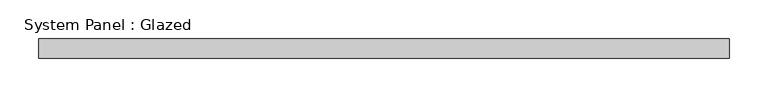
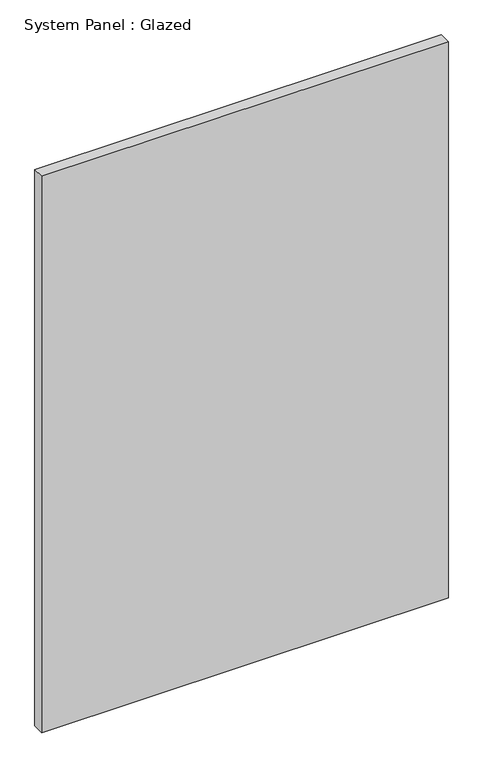
"""IFC4 building model written with IfcOpenShell, lengths in millimetres: plate geometry, System Panel : Glazed."""

from ifc_helpers import new_model, si_unit, origin, origin_with_axes, place, context, project, spatial, polyline, outline, extrude, source, transform, mapped, element, save


def system_panel_glazed_e669d95e(model_context):
    return source(origin(), model_context, "Body", "SweptSolid", [
        extrude(outline(polyline([(447.675, 19.05), (-447.675, 19.05), (-447.675, 44.45), (447.675, 44.45), (447.675, 19.05)])), origin_with_axes(), (0.0, 0.0, 1.0), 1295.1292854),
    ])


if __name__ == "__main__":
    model = new_model("IFC4")
    model_context = context("Model", 3, world=origin())
    ifc_project = project(units=[si_unit("LENGTHUNIT", "METRE", prefix="MILLI")], contexts=[model_context])
    site = spatial("IfcSite", under=ifc_project)
    building = spatial("IfcBuilding", under=site)
    placement = place(None, origin())
    system_panel_glazed_shape = system_panel_glazed_e669d95e(model_context)
    element("IfcPlate", 1, ObjectType="System Panel : Glazed", at=placement, inside=building, context=model_context, shape_type="MappedRepresentation", body=[
        mapped(system_panel_glazed_shape, transform((0.0, 0.0, 0.0), x_axis=(1.0, 0.0, 0.0), y_axis=(0.0, 1.0, 0.0), z_axis=(0.0, 0.0, 1.0))),
    ])
    save(model, "model.ifc")

# Revit data of these elements
# Type "System Panel : Glazed"
#   Construction Type Id = "GSP4R"
#   Analytic Construction = "1/8 in Pilkington single glazing"
#   Visual Light Transmittance = 0.9
#   Solar Heat Gain Coefficient = 0.86
#   Heat Transfer Coefficient (U) = 1.18115 BTU/(h·ft²·°F)
#   Define Thermal Properties by = 1
# Element 1 (IfcPlate, "System Panel : Glazed")
#   Materials on its faces: "Glass"
# Materials
#   "Glass": class "Glass", colour RGB 0 128 192, transparency 0.75, Description = "Soda Lime Glass", Cost = 0
